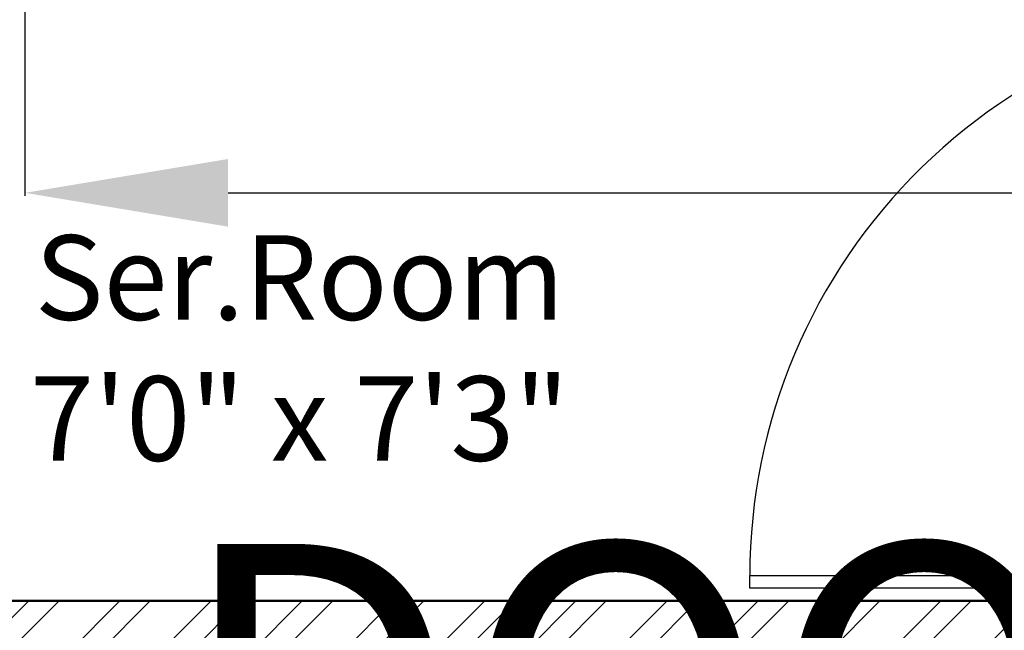
# Model space of a CAD drawing. Units: inches. Extents: x -90 to 536, y -553 to 299.
# Tile 4 of 27: x 96 to 155, y -430 to -394. Entities that reach past the tile are written whole.
import ezdxf

# ---------------------------------------------------------------- set-up
doc = ezdxf.new("R2010")
doc.units = ezdxf.units.IN
for name, color, linetype, lineweight in [('A-ANNO-DIMS', 2, 'Continuous', 18), ('A-AREA-IDEN', 7, 'Continuous', 18), ('A-DOOR', 4, 'Continuous', 25), ('A-WALL-PATT', 252, 'Continuous', 13), ('Outer Wall', 1, 'Continuous', 50)]:
    doc.layers.add(name, color=color, linetype=linetype, lineweight=lineweight)
doc.styles.get("Standard").update_dxf_attribs({"font": 'arial.ttf'})
doc.dimstyles.get("Standard").update_dxf_attribs({"dimtxt": 18, "dimasz": 12, "dimexe": 0.18, "dimexo": 0.0625, "dimgap": 0.09, "dimtad": 0, "dimtih": 1, "dimtoh": 1, "dimdec": 0, "dimzin": 0, "dimdsep": 46, "dimlunit": 3, "dimtxsty": 'Standard', "dimcen": 0.09, "dimadec": 0, "dimazin": 0, "dimtfac": 1, "dimtdec": 0, "dimtofl": 0, "dimtmove": 0, "dimatfit": 3, "dimfxl": 1, "dimtolj": 1, "dimtzin": 0, "dimarcsym": 0})

# ---------------------------------------------------------------- blocks, each defined once
blk = doc.blocks.new('DOOR-36-B')
for points in [[(37.5, 36), (37.5, 34.5), (36, 34.5), (36, 35.25), (34.5, 35.25), (34.5, 36)], [(0, 0.75), (0, 1.5), (34.5, 1.5), (34.5, 0.75)], [(37.5, 0), (37.5, 1.5), (36, 1.5), (36, 0.75), (34.5, 0.75), (34.5, 0)]]:
    blk.add_lwpolyline(points, close=True)
blk.add_arc((33.758, 1.5), 33.758, 88.7408, 180)
blk = doc.blocks.new('*D27')
at = {"layer": 'A-ANNO-DIMS', "color": 0, "lineweight": -2, "transparency": 16777216}
for p, q in [((49.132, -428.616), (49.132, -434.359)), ((86.632, -428.616), (86.632, -434.359)), ((61.132, -434.179), (74.632, -434.179)), ((86.632, -434.179), (98.632, -434.179))]:
    blk.add_line(p, q, dxfattribs=at)
at = {"layer": 'A-ANNO-DIMS', "color": 0, "transparency": 16777216}
for points in [[(61.132, -432.179), (61.132, -436.179), (49.132, -434.179)], [(74.632, -432.179), (74.632, -436.179), (86.632, -434.179)]]:
    blk.add_solid(points, dxfattribs=at)
at = {"layer": 'Defpoints', "color": 0, "transparency": 16777216}
for p in [(49.132, -428.554), (86.632, -428.554), (86.632, -434.179)]:
    blk.add_point(p, dxfattribs=at)
at = {"layer": 'A-ANNO-DIMS', "color": 0, "transparency": 16777216, "insert": (195.174, -434.179), "char_height": 18, "attachment_point": 5}
blk.add_mtext('\\A1;DOOR B 38 TYP.', dxfattribs=at)
blk = doc.blocks.new('*D28')
at = {"layer": 'A-ANNO-DIMS', "color": 0, "lineweight": -2, "transparency": 16777216}
for p, q in [((92.257, -392.554), (92.257, -380.554)), ((92.257, -380.554), (104.257, -380.554)), ((86.694, -392.554), (92.437, -392.554)), ((92.257, -416.554), (92.257, -404.554)), ((86.694, -428.554), (92.437, -428.554))]:
    blk.add_line(p, q, dxfattribs=at)
at = {"layer": 'A-ANNO-DIMS', "color": 0, "transparency": 16777216}
for points in [[(90.257, -404.554), (94.257, -404.554), (92.257, -392.554)], [(90.257, -416.554), (94.257, -416.554), (92.257, -428.554)]]:
    blk.add_solid(points, dxfattribs=at)
at = {"layer": 'Defpoints', "color": 0, "transparency": 16777216}
for p in [(86.632, -392.554), (92.257, -392.554), (86.632, -428.554)]:
    blk.add_point(p, dxfattribs=at)
at = {"layer": 'A-ANNO-DIMS', "color": 0, "transparency": 16777216, "insert": (148.15, -380.554), "char_height": 18, "attachment_point": 5}
blk.add_mtext('\\A1;36 TYP.', dxfattribs=at)
blk = doc.blocks.new('*D35')
at = {"layer": 'A-ANNO-DIMS', "color": 0, "lineweight": -2, "transparency": 16777216}
for p, q in [((233.194, -331.054), (239.837, -331.054)), ((239.657, -343.054), (239.657, -343.401)), ((239.657, -362.554), (239.657, -362.207)), ((233.194, -374.554), (239.837, -374.554))]:
    blk.add_line(p, q, dxfattribs=at)
at = {"layer": 'A-ANNO-DIMS', "color": 0, "transparency": 16777216}
for points in [[(237.657, -343.054), (241.657, -343.054), (239.657, -331.054)], [(237.657, -362.554), (241.657, -362.554), (239.657, -374.554)]]:
    blk.add_solid(points, dxfattribs=at)
at = {"layer": 'Defpoints', "color": 0, "transparency": 16777216}
for p in [(233.132, -331.054), (239.657, -331.054), (233.132, -374.554)]:
    blk.add_point(p, dxfattribs=at)
at = {"layer": 'A-ANNO-DIMS', "color": 0, "transparency": 16777216, "insert": (239.657, -352.804), "char_height": 18, "attachment_point": 5}
blk.add_mtext('\\A1;ENTRY DOOR 44 TYP.', dxfattribs=at)
blk = doc.blocks.new('*D51')
at = {"layer": 'A-ANNO-DIMS', "color": 0, "lineweight": -2, "transparency": 16777216}
for p, q in [((96.806, -393.34), (96.806, -404.606)), ((171.132, -393.34), (171.132, -404.606)), ((108.806, -404.426), (159.132, -404.426)), ((171.132, -404.426), (183.132, -404.426))]:
    blk.add_line(p, q, dxfattribs=at)
at = {"layer": 'A-ANNO-DIMS', "color": 0, "transparency": 16777216}
for points in [[(108.806, -402.426), (108.806, -406.426), (96.806, -404.426)], [(159.132, -402.426), (159.132, -406.426), (171.132, -404.426)]]:
    blk.add_solid(points, dxfattribs=at)
at = {"layer": 'Defpoints', "color": 0, "transparency": 16777216}
for p in [(96.806, -393.277), (171.132, -393.277), (171.132, -404.426)]:
    blk.add_point(p, dxfattribs=at)
at = {"layer": 'A-ANNO-DIMS', "color": 0, "transparency": 16777216, "insert": (274.99, -404.426), "char_height": 18, "attachment_point": 5}
blk.add_mtext('\\A1;SINGLE BED 74', dxfattribs=at)
blk = doc.blocks.new('*D54')
at = {"layer": 'A-ANNO-DIMS', "color": 0, "lineweight": -2, "transparency": 16777216}
for p, q in [((113.069, 249.446), (-2.848, 249.446)), ((-2.668, 237.446), (-2.668, -117.767)), ((-2.668, -491.554), (-2.668, -136.34)), ((38.069, -503.554), (-2.848, -503.554))]:
    blk.add_line(p, q, dxfattribs=at)
at = {"layer": 'A-ANNO-DIMS', "color": 0, "transparency": 16777216}
for points in [[(-4.668, 237.446), (-0.668, 237.446), (-2.668, 249.446)], [(-4.668, -491.554), (-0.668, -491.554), (-2.668, -503.554)]]:
    blk.add_solid(points, dxfattribs=at)
at = {"layer": 'Defpoints', "color": 0, "transparency": 16777216}
for p in [(-2.668, 249.446), (113.132, 249.446), (38.132, -503.554)]:
    blk.add_point(p, dxfattribs=at)
at = {"layer": 'A-ANNO-DIMS', "color": 0, "transparency": 16777216, "insert": (-2.668, -127.054), "char_height": 18, "attachment_point": 5}
blk.add_mtext('\\A1;753', dxfattribs=at)

msp = doc.modelspace()

# ---------------------------------------------------------------- hatches: boundary and pattern name
at = {"layer": 'A-WALL-PATT'}
h = msp.add_hatch(dxfattribs=at)
h.set_pattern_fill('ANSI32', color=256, scale=0.4)
h.set_pattern_definition([(45, (-88.8105, -603.6155), (-2.694077, 2.694077), []), (45, (-87.0145, -603.6155), (-2.694077, 2.694077), [])])
h.paths.add_polyline_path([(285.1317, 246.4462), (131.1317, 246.4462), (131.1317, 237.4462), (285.1317, 237.4462)])
h.paths.add_polyline_path([(122.1317, 237.4462), (113.1317, 237.4462), (113.1317, 152.4462), (122.1317, 152.4462), (122.1317, 166.4704)])
h.paths.add_polyline_path([(303.1317, 237.4462), (294.1317, 237.4462), (294.1317, 152.4462), (303.1317, 152.4462)])
h.paths.add_polyline_path([(47.1317, 91.9277), (38.1317, 91.9277), (38.1317, -6.5538), (77.1317, -6.5538), (77.1317, 2.4462), (70.5655, 2.4462), (47.1317, 2.4462)])
h.paths.add_polyline_path([(83.052, -61.5538), (47.1317, -61.5538), (47.1317, -24.5538), (38.1317, -24.5538), (38.1317, -70.5538), (74.052, -70.5538), (74.052, -223.5538), (38.1317, -223.5538), (38.1317, -503.5538), (92.1317, -503.5538), (92.1317, -437.5538), (191.1317, -437.5538), (191.1317, -428.5538), (83.1317, -428.5538), (83.1317, -494.5538), (47.1317, -494.5538), (47.1317, -232.5538), (83.052, -232.5538), (83.052, -70.5538)])
h.paths.add_polyline_path([(407.1317, -63.5538), (381.1317, -63.5538), (381.1317, 91.9277), (372.1317, 91.9277), (372.1317, 32.8805), (372.1317, -63.5538), (306.5745, -63.5538), (237.1317, -63.5538), (237.1317, -38.5538), (233.1317, -38.5538), (233.1317, -71.5538), (398.1317, -71.5538), (398.1317, -152.5538), (233.1317, -152.5538), (233.1317, -161.5538), (398.1317, -161.5538), (398.1317, -368.5538), (233.1317, -368.5538), (233.1317, -377.5538), (407.1317, -377.5538), (407.1317, -161.5538)])
h.paths.add_polyline_path([(261.1317, -422.5538), (252.1317, -422.5538), (252.1317, -428.5538), (233.1317, -428.5538), (233.1317, -437.5538), (261.1317, -437.5538)])
h.paths.add_polyline_path([(191.1317, -368.5538), (180.1317, -368.5538), (180.1317, -335.5538), (131.5919, -335.5538), (131.5919, -344.5538), (171.1317, -344.5538), (171.1317, -392.5538), (180.1317, -392.5538), (180.1317, -377.5538), (191.1317, -377.5538)], flags=17)
h.paths.add_polyline_path([(180.1317, -223.5538), (152.1317, -223.5538), (152.1317, -227.5538), (176.1317, -227.5538), (176.1317, -335.5538), (180.1317, -335.5538)], flags=17)
h.paths.add_polyline_path([(131.5919, -335.5538), (83.1317, -335.5538), (83.1317, -339.5538), (83.1317, -392.5538), (87.1317, -392.5538), (87.1317, -339.5538), (131.5919, -339.5538)], flags=17)
h.paths.add_polyline_path([(197.1317, 2.4462), (77.1317, 2.4462), (77.1317, -1.5538), (113.1317, -1.5538), (113.1317, -71.5538), (181.1317, -71.5538), (181.1317, -67.5538), (117.1317, -67.5538), (117.1317, -1.5538), (177.1317, -1.5538), (177.1317, -37.5538), (181.1317, -37.5538), (181.1317, -1.5538), (197.1317, -1.5538)])
h.paths.add_polyline_path([(173.1317, 138.4462), (122.1317, 138.4462), (122.1317, 134.4462), (173.1317, 134.4462)])
h.paths.add_polyline_path([(213.1317, 237.4462), (209.1317, 237.4462), (209.1317, 134.4462), (233.1317, 134.4462), (233.1317, 68.8889), (233.1317, -2.5538), (237.1317, -2.5538), (237.1317, 134.4462), (258.1317, 134.4462), (258.1317, 138.4462), (213.1317, 138.4462)])

# ---------------------------------------------------------------- linework, layer by layer
at = {"layer": 'Outer Wall'}
msp.add_line((191.1317, -428.5538), (83.1317, -428.5538), dxfattribs=at)

# ---------------------------------------------------------------- block references
at = {"layer": 'A-DOOR'}
msp.add_blockref('DOOR-36-B', (139.6317, -428.5538), dxfattribs=at)

# ---------------------------------------------------------------- texts
at = {"layer": 'A-AREA-IDEN', "insert": (137.7038, -406.933), "char_height": 5, "attachment_point": 3}
msp.add_mtext_dynamic_manual_height_columns('\\pxqc;{\\fTimes New Roman|b0|i0|c0|p18;Ser.Room\\P7\'0" x 7\'3"}', width=49.342153, gutter_width=12.5, heights=[0], dxfattribs=at)

# ---------------------------------------------------------------- dimensions: what is measured, and where the dimension line sits
at = {"layer": 'A-ANNO-DIMS'}
dim = msp.add_linear_dim(base=(-2.6677, 249.4462), p1=(38.1317, -503.5538), p2=(113.1317, 249.4462), angle=90, dimstyle='Standard', override={"dimdec": 0, "dimlfac": 1, "dimrnd": 0, "dimzin": 0, "dimdsep": 46, "dimlunit": 2}, dxfattribs=at)
dim.commit()
dim.dimension.update_dxf_attribs({"geometry": '*D54', "text_midpoint": (-2.6677, -127.0538)})
for base, p1, p2, text, picture, middle in [((239.6567404714, -331.0537825705), (233.1317404714, -374.5537825705), (233.1317404714, -331.0537825705), 'ENTRY DOOR <> TYP.', '*D35', (239.6567404714, -352.8037825705)), ((92.2567, -392.5538), (86.6317, -428.5538), (86.6317, -392.5538), '<> TYP.', '*D28', (148.1496, -380.5538))]:
    dim = msp.add_linear_dim(base=base, p1=p1, p2=p2, angle=90, text=text, dimstyle='Standard', override={"dimdec": 0, "dimlfac": 1, "dimrnd": 0, "dimzin": 0, "dimdsep": 46, "dimlunit": 2}, dxfattribs=at)
    dim.commit()
    dim.dimension.update_dxf_attribs({"geometry": picture, "text_midpoint": middle})
for base, p1, p2, text, picture, middle in [((171.1317, -404.4263), (96.8056, -393.2773), (171.1317, -393.2773), 'SINGLE BED <>', '*D51', (274.9898, -404.4263)), ((86.6317404714, -434.1787825705), (49.1317404714, -428.5537825705), (86.6317404714, -428.5537825705), 'DOOR B <> TYP.', '*D27', (195.1739914946, -434.1787825705))]:
    dim = msp.add_linear_dim(base=base, p1=p1, p2=p2, text=text, dimstyle='Standard', override={"dimdec": 0, "dimlfac": 1, "dimrnd": 0, "dimzin": 0, "dimdsep": 46, "dimlunit": 2}, dxfattribs=at)
    dim.commit()
    dim.dimension.update_dxf_attribs({"geometry": picture, "text_midpoint": middle})

doc.saveas('drawing.dxf')
